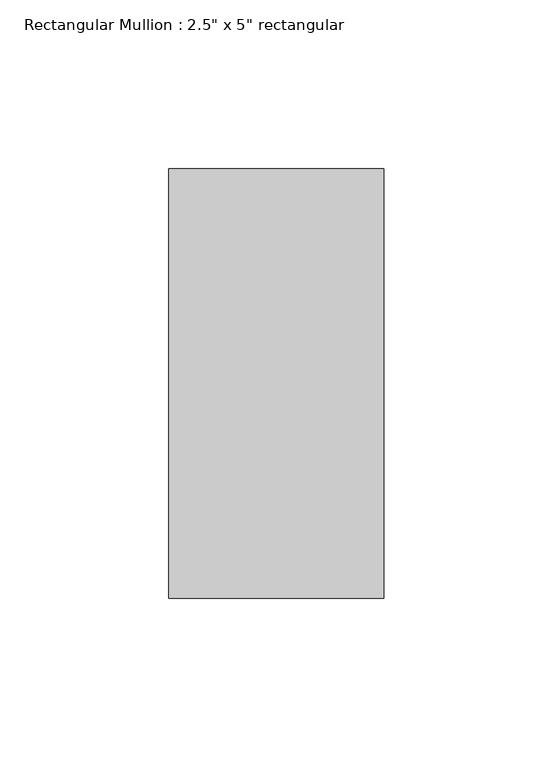
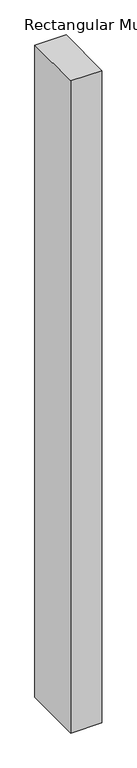
"""IFC4 building model written with IfcOpenShell, lengths in millimetres: member geometry."""

from ifc_helpers import new_model, si_unit, frame, origin, place, context, project, spatial, polyline, outline, extrude, source, transform, mapped, element, save


def member_48accb65(model_context):
    return source(origin(), model_context, "Body", "SweptSolid", [
        extrude(outline(polyline([(0.0, 63.5), (0.0, -63.5), (-63.5, -63.5), (-63.5, 63.5), (0.0, 63.5)])), frame((0.0, 0.0, -1408.1788335), z_axis=(0.0, 0.0, 1.0), x_axis=(1.0, 0.0, 0.0)), (0.0, 0.0, 1.0), 1408.1788335),
    ])


if __name__ == "__main__":
    model = new_model("IFC4")
    model_context = context("Model", 3, world=origin())
    ifc_project = project(units=[si_unit("LENGTHUNIT", "METRE", prefix="MILLI")], contexts=[model_context])
    site = spatial("IfcSite", under=ifc_project)
    building = spatial("IfcBuilding", under=site)
    placement = place(None, origin())
    member_shape = member_48accb65(model_context)
    element("IfcMember", 1, ObjectType="Rectangular Mullion : 2.5\" x 5\" rectangular", at=placement, inside=building, context=model_context, shape_type="MappedRepresentation", body=[
        mapped(member_shape, transform((0.0, 0.0, 0.0), x_axis=(1.0, 0.0, 0.0), y_axis=(0.0, 1.0, 0.0), z_axis=(0.0, 0.0, 1.0))),
    ])
    save(model, "model.ifc")

# Revit data of these elements
# Type "Rectangular Mullion : 2.5\" x 5\" rectangular"
#   built-in parameter 1007304 = 0.416667 (stored number, unit not read)
#   built-in parameter 1007301 = 0.104167 (stored number, unit not read)
#   built-in parameter 1007300 = 0.104167 (stored number, unit not read)
# Element 1 (IfcMember, "Rectangular Mullion : 2.5\" x 5\" rectangular")
#   Materials on its faces: "Aluminum"
# Materials
#   "Aluminum": class "Metal", colour RGB 247 247 247, transparency 0, Description = "Aluminum 6061", Cost = 0
